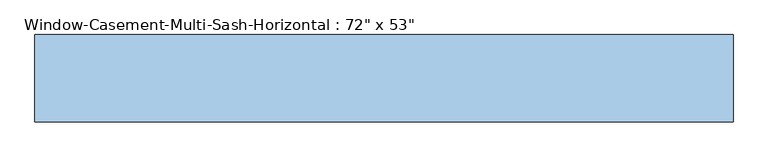
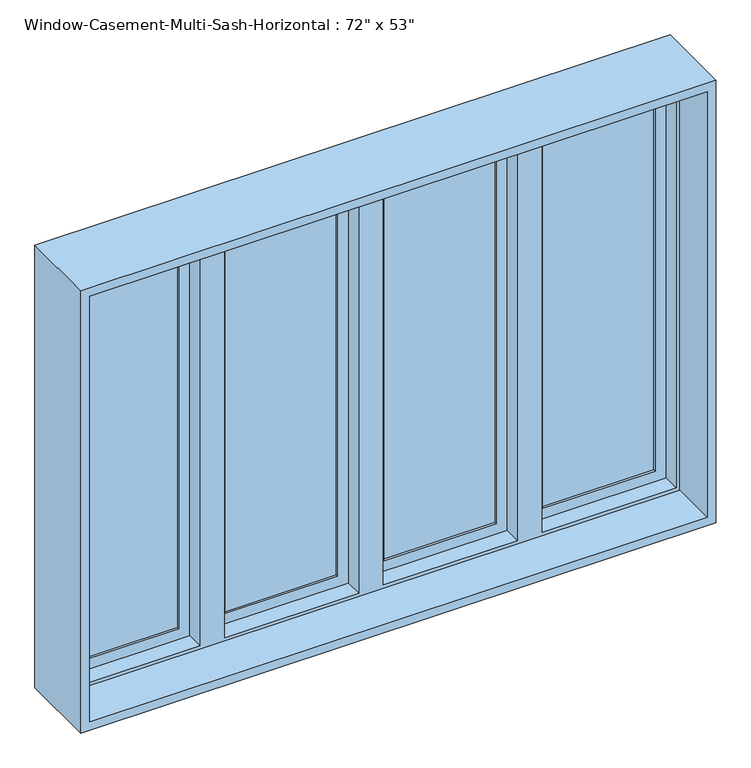
"""IFC4 building model written with IfcOpenShell, lengths in millimetres: window geometry."""

from ifc_helpers import new_model, si_unit, frame, origin, place, context, project, spatial, polyline, outline, extrude, faceted_brep, source, transform, mapped, element, save


def window_5487fb6d(model_context):
    return source(origin(), model_context, "Body", "SolidModel", [
        extrude(outline(polyline([(2235.2, 482.6), (939.8, 482.6), (939.8, 889.0), (2235.2, 889.0), (2235.2, 482.6)]), holes=[polyline([(2193.3296875, 847.1296875), (981.6703125, 847.1296875), (981.6703125, 524.4703125), (2193.3296875, 524.4703125), (2193.3296875, 847.1296875)])]), frame((0.0, 73.025, 0.0), z_axis=(0.0, 1.0, 0.0), x_axis=(0.0, 0.0, 1.0)), (0.0, 0.0, 1.0), 31.75),
        extrude(outline(polyline([(2235.2, -889.0), (939.8, -889.0), (939.8, -482.6), (2235.2, -482.6), (2235.2, -889.0)]), holes=[polyline([(2193.3296875, -524.4703125), (981.6703125, -524.4703125), (981.6703125, -847.1296875), (2193.3296875, -847.1296875), (2193.3296875, -524.4703125)])]), frame((0.0, 73.025, 0.0), z_axis=(0.0, 1.0, 0.0), x_axis=(0.0, 0.0, 1.0)), (0.0, 0.0, 1.0), 31.75),
        extrude(outline(polyline([(-524.4703125, 98.425), (-524.4703125, 92.075), (-847.1296875, 92.075), (-847.1296875, 98.425), (-524.4703125, 98.425)])), frame((0.0, 0.0, 981.6703125), z_axis=(0.0, 0.0, 1.0), x_axis=(1.0, 0.0, 0.0)), (0.0, 0.0, 1.0), 1211.659375),
        extrude(outline(polyline([(-524.4703125, 85.725), (-524.4703125, 79.375), (-847.1296875, 79.375), (-847.1296875, 85.725), (-524.4703125, 85.725)])), frame((0.0, 0.0, 981.6703125), z_axis=(0.0, 0.0, 1.0), x_axis=(1.0, 0.0, 0.0)), (0.0, 0.0, 1.0), 1211.659375),
        extrude(outline(polyline([(847.1296875, 98.425), (847.1296875, 92.075), (524.4703125, 92.075), (524.4703125, 98.425), (847.1296875, 98.425)])), frame((0.0, 0.0, 981.6703125), z_axis=(0.0, 0.0, 1.0), x_axis=(1.0, 0.0, 0.0)), (0.0, 0.0, 1.0), 1211.659375),
        extrude(outline(polyline([(847.1296875, 85.725), (847.1296875, 79.375), (524.4703125, 79.375), (524.4703125, 85.725), (847.1296875, 85.725)])), frame((0.0, 0.0, 981.6703125), z_axis=(0.0, 0.0, 1.0), x_axis=(1.0, 0.0, 0.0)), (0.0, 0.0, 1.0), 1211.659375),
        extrude(outline(polyline([(-67.2703125, 98.425), (-67.2703125, 92.075), (-389.9296875, 92.075), (-389.9296875, 98.425), (-67.2703125, 98.425)])), frame((0.0, 0.0, 981.6703125), z_axis=(0.0, 0.0, 1.0), x_axis=(1.0, 0.0, 0.0)), (0.0, 0.0, 1.0), 1211.659375),
        extrude(outline(polyline([(-67.2703125, 85.725), (-67.2703125, 79.375), (-389.9296875, 79.375), (-389.9296875, 85.725), (-67.2703125, 85.725)])), frame((0.0, 0.0, 981.6703125), z_axis=(0.0, 0.0, 1.0), x_axis=(1.0, 0.0, 0.0)), (0.0, 0.0, 1.0), 1211.659375),
        extrude(outline(polyline([(389.9296875, 98.425), (389.9296875, 92.075), (67.2703125, 92.075), (67.2703125, 98.425), (389.9296875, 98.425)])), frame((0.0, 0.0, 981.6703125), z_axis=(0.0, 0.0, 1.0), x_axis=(1.0, 0.0, 0.0)), (0.0, 0.0, 1.0), 1211.659375),
        extrude(outline(polyline([(389.9296875, 85.725), (389.9296875, 79.375), (67.2703125, 79.375), (67.2703125, 85.725), (389.9296875, 85.725)])), frame((0.0, 0.0, 981.6703125), z_axis=(0.0, 0.0, 1.0), x_axis=(1.0, 0.0, 0.0)), (0.0, 0.0, 1.0), 1211.659375),
        faceted_brep([(-482.6, 73.025, 2235.2), (-889.0, 73.025, 2235.2), (-889.0, 114.3, 2235.2), (889.0, 114.3, 2235.2), (889.0, 73.025, 2235.2), (482.6, 73.025, 2235.2), (482.6, 111.125, 2235.2), (431.8, 111.125, 2235.2), (431.8, 73.025, 2235.2), (25.4, 73.025, 2235.2), (25.4, 111.125, 2235.2), (-25.4, 111.125, 2235.2), (-25.4, 73.025, 2235.2), (-431.8, 73.025, 2235.2), (-431.8, 111.125, 2235.2), (-482.6, 111.125, 2235.2), (-878.8796875, 22.225, 2225.0796875), (-878.8796875, 73.025, 2225.0796875), (-492.7203125, 73.025, 2225.0796875), (-492.7203125, 22.225, 2225.0796875), (878.8796875, 73.025, 2225.0796875), (878.8796875, 22.225, 2225.0796875), (492.7203125, 22.225, 2225.0796875), (492.7203125, 73.025, 2225.0796875), (-421.6796875, 73.025, 2225.0796875), (-35.5203125, 73.025, 2225.0796875), (-35.5203125, 22.225, 2225.0796875), (-421.6796875, 22.225, 2225.0796875), (35.5203125, 73.025, 2225.0796875), (421.6796875, 73.025, 2225.0796875), (421.6796875, 22.225, 2225.0796875), (35.5203125, 22.225, 2225.0796875), (-889.0, -114.3, 2235.2), (-889.0, 22.225, 2235.2), (889.0, 22.225, 2235.2), (889.0, -114.3, 2235.2), (-914.4, 114.3, 2260.6), (-914.4, -114.3, 2260.6), (914.4, -114.3, 2260.6), (914.4, 114.3, 2260.6), (889.0, 114.3, 939.8), (889.0, 73.025, 939.8), (878.8796875, 73.025, 949.9203125), (878.8796875, 22.225, 949.9203125), (889.0, 22.225, 939.8), (889.0, -114.3, 939.8), (914.4, -114.3, 914.4), (914.4, 114.3, 914.4), (482.6, 73.025, 939.8), (-889.0, 114.3, 939.8), (-889.0, 73.025, 939.8), (-482.6, 73.025, 939.8), (-482.6, 111.125, 939.8), (-431.8, 111.125, 939.8), (-431.8, 73.025, 939.8), (-25.4, 73.025, 939.8), (-25.4, 111.125, 939.8), (25.4, 111.125, 939.8), (25.4, 73.025, 939.8), (431.8, 73.025, 939.8), (431.8, 111.125, 939.8), (482.6, 111.125, 939.8), (492.7203125, 73.025, 949.9203125), (492.7203125, 22.225, 949.9203125), (-878.8796875, 73.025, 949.9203125), (-878.8796875, 22.225, 949.9203125), (-492.7203125, 22.225, 949.9203125), (-492.7203125, 73.025, 949.9203125), (-35.5203125, 73.025, 949.9203125), (-421.6796875, 73.025, 949.9203125), (-421.6796875, 22.225, 949.9203125), (-35.5203125, 22.225, 949.9203125), (421.6796875, 73.025, 949.9203125), (35.5203125, 73.025, 949.9203125), (35.5203125, 22.225, 949.9203125), (421.6796875, 22.225, 949.9203125), (-889.0, 22.225, 939.8), (-889.0, -114.3, 939.8), (-914.4, -114.3, 914.4), (-914.4, 114.3, 914.4)], [[[0, 1, 2, 3, 4, 5, 6, 7, 8, 9, 10, 11, 12, 13, 14, 15]], [[16, 17, 18, 19]], [[20, 21, 22, 23]], [[24, 25, 26, 27]], [[28, 29, 30, 31]], [[32, 33, 34, 35]], [[36, 37, 38, 39]], [[4, 3, 40, 41]], [[21, 20, 42, 43]], [[35, 34, 44, 45]], [[39, 38, 46, 47]], [[48, 41, 40, 49, 50, 51, 52, 53, 54, 55, 56, 57, 58, 59, 60, 61]], [[43, 42, 62, 63]], [[64, 65, 66, 67]], [[68, 69, 70, 71]], [[72, 73, 74, 75]], [[45, 44, 76, 77]], [[47, 46, 78, 79]], [[2, 1, 50, 49]], [[4, 41, 48, 5], [20, 23, 62, 42]], [[50, 1, 0, 51], [64, 67, 18, 17]], [[12, 55, 54, 13], [69, 68, 25, 24]], [[8, 59, 58, 9], [73, 72, 29, 28]], [[17, 16, 65, 64]], [[44, 34, 33, 76], [16, 19, 66, 65], [27, 26, 71, 70], [31, 30, 75, 74], [21, 43, 63, 22]], [[33, 32, 77, 76]], [[38, 37, 78, 46], [32, 35, 45, 77]], [[37, 36, 79, 78]], [[36, 39, 47, 79], [3, 2, 49, 40]], [[18, 67, 66, 19]], [[69, 24, 27, 70]], [[53, 14, 13, 54]], [[14, 53, 52, 15]], [[15, 52, 51, 0]], [[25, 68, 71, 26]], [[73, 28, 31, 74]], [[57, 10, 9, 58]], [[10, 57, 56, 11]], [[11, 56, 55, 12]], [[6, 61, 60, 7]], [[7, 60, 59, 8]], [[29, 72, 75, 30]], [[62, 23, 22, 63]], [[61, 6, 5, 48]]]),
        extrude(outline(polyline([(2235.2, 25.4), (939.8, 25.4), (939.8, 431.8), (2235.2, 431.8), (2235.2, 25.4)]), holes=[polyline([(2193.3296875, 389.9296875), (981.6703125, 389.9296875), (981.6703125, 67.2703125), (2193.3296875, 67.2703125), (2193.3296875, 389.9296875)])]), frame((0.0, 73.025, 0.0), z_axis=(0.0, 1.0, 0.0), x_axis=(0.0, 0.0, 1.0)), (0.0, 0.0, 1.0), 31.75),
        extrude(outline(polyline([(2235.2, -431.8), (939.8, -431.8), (939.8, -25.4), (2235.2, -25.4), (2235.2, -431.8)]), holes=[polyline([(2193.3296875, -67.2703125), (981.6703125, -67.2703125), (981.6703125, -389.9296875), (2193.3296875, -389.9296875), (2193.3296875, -67.2703125)])]), frame((0.0, 73.025, 0.0), z_axis=(0.0, 1.0, 0.0), x_axis=(0.0, 0.0, 1.0)), (0.0, 0.0, 1.0), 31.75),
    ])


if __name__ == "__main__":
    model = new_model("IFC4")
    model_context = context("Model", 3, world=origin())
    ifc_project = project(units=[si_unit("LENGTHUNIT", "METRE", prefix="MILLI")], contexts=[model_context])
    site = spatial("IfcSite", under=ifc_project)
    building = spatial("IfcBuilding", under=site)
    placement = place(None, origin())
    window_shape = window_5487fb6d(model_context)
    element("IfcWindow", 1, ObjectType="Window-Casement-Multi-Sash-Horizontal : 72\" x 53\"", at=placement, inside=building, context=model_context, shape_type="MappedRepresentation", body=[
        mapped(window_shape, transform((0.0, 0.0, 0.0), x_axis=(1.0, 0.0, 0.0), y_axis=(0.0, 1.0, 0.0), z_axis=(0.0, 0.0, 1.0))),
    ])
    save(model, "model.ifc")

# Revit data of these elements
# Type "Window-Casement-Multi-Sash-Horizontal : 72\" x 53\""
#   Type Mark = "24"
#   Fire Rating = "0.5h"
#   Assembly Code = "B2020100"
#   Analytic Construction = "Double glazing - domestic"
#   Window Inset [instance default] = 0' - 0 5/8"
#   Wall Thickness [instance default] = 0' - 6"
#   Visual Light Transmittance = 0.81
#   Thermal Resistance (R) = 1.8146 (h·ft²·°F)/BTU
#   Solar Heat Gain Coefficient = 0.76
#   Rough Width = 6' - 0 1/2"
#   Rough Height = 4' - 5 1/2"
#   Open Window Width = 1' - 6"
#   Heat Transfer Coefficient (U) = 0.5511 BTU/(h·ft²·°F)
#   Height = 4' - 5"
#   Frame Gap 3 [instance default] = 0' - 1 83/128"
#   Frame Gap 2 [instance default] = 0' - 0 5/8"
#   Frame Gap 1 = 0' - 1 51/128"
#   Default Sill Height = 3' - 0"
#   Width = 6' - 0"
#   Frame Material = Metal - Aluminum
#   Glass Panel Material = Glass
#   Wall Closure = (empty or 0)
# Element 1 (IfcWindow, "Window-Casement-Multi-Sash-Horizontal : 72\" x 53\"")
#   Wall Thickness = 0' - 9"
#   Materials on its faces: "Metal - Aluminum", "Glass"
# Materials
#   "Metal - Aluminum": class "Metal", colour RGB 247 247 247, transparency 0
#   "Glass": class "Glass", colour RGB 0 128 192, transparency 0.75, Description = "Soda Lime Glass", Cost = 0
